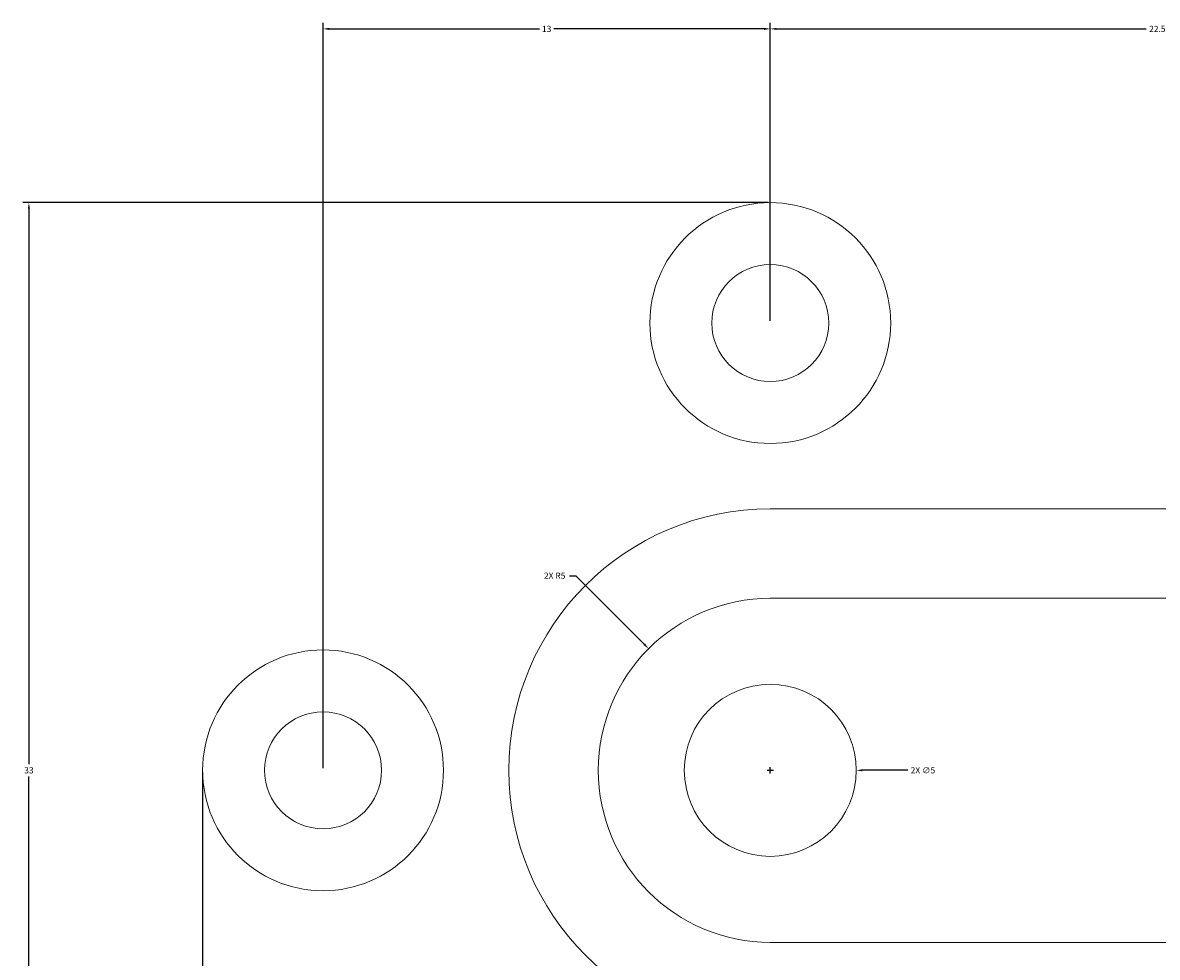
# Model space of a CAD drawing. Units: millimetres. Extents: x 3243.8 to 3309.8, y 1625.7 to 1669.2.
# Tile 2 of 3: x 3243.8 to 3276.8, y 1642 to 1669.2. Entities that reach past the tile are written whole.
import ezdxf

# ---------------------------------------------------------------- set-up
doc = ezdxf.new("R2010")
doc.units = ezdxf.units.MM
doc.layers.add('M-CONS', color=8, linetype='Continuous', lineweight=18)
doc.layers.add('M-DIMS', color=2, linetype='Continuous', lineweight=18)
doc.styles.get("Standard").update_dxf_attribs({"font": 'arial.ttf'})
doc.dimstyles.get("Standard").update_dxf_attribs({"dimtxt": 0.18, "dimasz": 0.18, "dimexe": 0.18, "dimexo": 0.0625, "dimgap": 0.09, "dimtad": 0, "dimtih": 1, "dimtoh": 1, "dimdec": 4, "dimzin": 0, "dimdsep": 46, "dimtxsty": 'Standard', "dimcen": 0.09, "dimadec": 0, "dimazin": 0, "dimtfac": 1, "dimtdec": 4, "dimtofl": 0, "dimtmove": 0, "dimatfit": 3, "dimfxl": 1, "dimtolj": 1, "dimtzin": 0, "dimarcsym": 0})

# ---------------------------------------------------------------- blocks, each defined once
blk = doc.blocks.new('CBORE-7-BORE-3.4')
for centre, radius in [((3.5, 3.5), 3.5), ((3.5, 3.5, -1), 1.7)]:
    blk.add_circle(centre, radius)
blk = doc.blocks.new('*D2')
at = {"layer": 'Defpoints', "color": 0, "transparency": 16777216}
for p in [(3249.045, 1647.47), (3304.545, 1647.47), (3304.545, 1625.92)]:
    blk.add_point(p, dxfattribs=at)
at = {"layer": 'M-DIMS', "color": 0, "lineweight": -2, "transparency": 16777216}
for p, q in [((3249.045, 1647.407), (3249.045, 1625.74)), ((3304.545, 1647.407), (3304.545, 1625.74)), ((3249.225, 1625.92), (3276.47, 1625.92)), ((3304.365, 1625.92), (3277.119, 1625.92))]:
    blk.add_line(p, q, dxfattribs=at)
at = {"layer": 'M-DIMS', "color": 0, "transparency": 16777216}
for points in [[(3249.225, 1625.95), (3249.225, 1625.89), (3249.045, 1625.92)], [(3304.365, 1625.95), (3304.365, 1625.89), (3304.545, 1625.92)]]:
    blk.add_solid(points, dxfattribs=at)
at = {"layer": 'M-DIMS', "color": 0, "transparency": 16777216, "insert": (3276.795, 1625.92), "char_height": 0.18, "attachment_point": 5}
blk.add_mtext('\\A1;55.5', dxfattribs=at)
blk = doc.blocks.new('*D3')
at = {"layer": 'Defpoints', "color": 0, "transparency": 16777216}
for p in [(3243.995, 1663.97), (3265.545, 1663.97), (3265.545, 1630.97)]:
    blk.add_point(p, dxfattribs=at)
at = {"layer": 'M-DIMS', "color": 0, "lineweight": -2, "transparency": 16777216}
for p, q in [((3265.482, 1663.97), (3243.815, 1663.97)), ((3243.995, 1663.79), (3243.995, 1647.652)), ((3243.995, 1631.15), (3243.995, 1647.288)), ((3265.482, 1630.97), (3243.815, 1630.97))]:
    blk.add_line(p, q, dxfattribs=at)
at = {"layer": 'M-DIMS', "color": 0, "transparency": 16777216}
for points in [[(3243.965, 1663.79), (3244.025, 1663.79), (3243.995, 1663.97)], [(3243.965, 1631.15), (3244.025, 1631.15), (3243.995, 1630.97)]]:
    blk.add_solid(points, dxfattribs=at)
at = {"layer": 'M-DIMS', "color": 0, "transparency": 16777216, "insert": (3243.995, 1647.47), "char_height": 0.18, "attachment_point": 5}
blk.add_mtext('\\A1;33', dxfattribs=at)
blk = doc.blocks.new('*D4')
at = {"layer": 'Defpoints', "color": 0, "transparency": 16777216}
for p in [(3265.545, 1669.02), (3265.545, 1660.47), (3252.545, 1647.47)]:
    blk.add_point(p, dxfattribs=at)
at = {"layer": 'M-DIMS', "color": 0, "lineweight": -2, "transparency": 16777216}
for p, q in [((3252.545, 1647.532), (3252.545, 1669.2)), ((3265.545, 1660.532), (3265.545, 1669.2)), ((3252.725, 1669.02), (3258.834, 1669.02)), ((3265.365, 1669.02), (3259.255, 1669.02))]:
    blk.add_line(p, q, dxfattribs=at)
at = {"layer": 'M-DIMS', "color": 0, "transparency": 16777216}
for points in [[(3252.725, 1669.05), (3252.725, 1668.99), (3252.545, 1669.02)], [(3265.365, 1669.05), (3265.365, 1668.99), (3265.545, 1669.02)]]:
    blk.add_solid(points, dxfattribs=at)
at = {"layer": 'M-DIMS', "color": 0, "transparency": 16777216, "insert": (3259.045, 1669.02), "char_height": 0.18, "attachment_point": 5}
blk.add_mtext('\\A1;13', dxfattribs=at)
blk = doc.blocks.new('*D5')
at = {"layer": 'Defpoints', "color": 0, "transparency": 16777216}
for p in [(3288.045, 1669.02), (3265.545, 1660.47), (3288.045, 1660.47)]:
    blk.add_point(p, dxfattribs=at)
at = {"layer": 'M-DIMS', "color": 0, "lineweight": -2, "transparency": 16777216}
for p, q in [((3265.545, 1660.532), (3265.545, 1669.2)), ((3288.045, 1660.532), (3288.045, 1669.2)), ((3265.725, 1669.02), (3276.469, 1669.02)), ((3287.865, 1669.02), (3277.121, 1669.02))]:
    blk.add_line(p, q, dxfattribs=at)
at = {"layer": 'M-DIMS', "color": 0, "transparency": 16777216}
for points in [[(3265.725, 1669.05), (3265.725, 1668.99), (3265.545, 1669.02)], [(3287.865, 1669.05), (3287.865, 1668.99), (3288.045, 1669.02)]]:
    blk.add_solid(points, dxfattribs=at)
at = {"layer": 'M-DIMS', "color": 0, "transparency": 16777216, "insert": (3276.795, 1669.02), "char_height": 0.18, "attachment_point": 5}
blk.add_mtext('\\A1;22.5', dxfattribs=at)
blk = doc.blocks.new('*D8')
at = {"layer": 'Defpoints', "color": 0, "transparency": 16777216}
for p in [(3262.009, 1651.006), (3265.545, 1647.47)]:
    blk.add_point(p, dxfattribs=at)
at = {"layer": 'M-DIMS', "color": 0, "lineweight": -2, "transparency": 16777216}
for p, q in [((3259.708, 1653.127), (3259.888, 1653.127)), ((3259.888, 1653.127), (3261.882, 1651.133)), ((3265.455, 1647.47), (3265.635, 1647.47)), ((3265.545, 1647.38), (3265.545, 1647.56))]:
    blk.add_line(p, q, dxfattribs=at)
at = {"layer": 'M-DIMS', "color": 0, "transparency": 16777216}
blk.add_solid([(3261.903, 1651.154), (3261.861, 1651.112), (3262.009, 1651.006)], dxfattribs=at)
at = {"layer": 'M-DIMS', "color": 0, "transparency": 16777216, "insert": (3259.277, 1653.127), "char_height": 0.18, "attachment_point": 5}
blk.add_mtext('\\A1;2X R5', dxfattribs=at)
blk = doc.blocks.new('*D11')
at = {"layer": 'Defpoints', "color": 0, "transparency": 16777216}
for p in [(3263.045, 1647.47), (3268.045, 1647.47)]:
    blk.add_point(p, dxfattribs=at)
at = {"layer": 'M-DIMS', "color": 0, "lineweight": -2, "transparency": 16777216}
for p, q in [((3265.455, 1647.47), (3265.635, 1647.47)), ((3265.545, 1647.38), (3265.545, 1647.56)), ((3269.545, 1647.47), (3268.225, 1647.47))]:
    blk.add_line(p, q, dxfattribs=at)
at = {"layer": 'M-DIMS', "color": 0, "transparency": 16777216}
blk.add_solid([(3268.225, 1647.5), (3268.225, 1647.44), (3268.045, 1647.47)], dxfattribs=at)
at = {"layer": 'M-DIMS', "color": 0, "transparency": 16777216, "insert": (3269.982, 1647.47), "char_height": 0.18, "attachment_point": 5}
blk.add_mtext('\\A1;2X ∅5', dxfattribs=at)

msp = doc.modelspace()

# ---------------------------------------------------------------- linework, layer by layer
at = {"layer": 'M-CONS'}
for points in [[(3265.545, 1655.07), (3288.045, 1655.07, -1), (3288.045, 1639.87), (3265.545, 1639.87, -1)], [(3288.045, 1652.47), (3265.545, 1652.47, 1), (3265.545, 1642.47), (3288.045, 1642.47, 1)]]:
    msp.add_lwpolyline(points, format="xyb", close=True, dxfattribs=at)
for centre, radius in [((3265.545, 1660.47), 3.5), ((3265.545, 1660.47, -1), 1.7), ((3252.545, 1647.47), 3.5), ((3265.545, 1647.47), 2.5), ((3252.545, 1647.47, -1), 1.7)]:
    msp.add_circle(centre, radius, dxfattribs=at)

# ---------------------------------------------------------------- block references
for p in [(3262.045, 1656.97), (3249.045, 1643.97)]:
    msp.add_blockref('CBORE-7-BORE-3.4', p, dxfattribs=at)

# ---------------------------------------------------------------- dimensions: what is measured, and where the dimension line sits
at = {"layer": 'M-DIMS'}
for base, p1, p2, override, picture, middle in [((3265.545, 1669.02), (3252.545, 1647.47), (3265.545, 1660.47), {"dimdec": 0, "dimlfac": 1, "dimrnd": 0, "dimzin": 0, "dimdsep": 46, "dimlunit": 2}, '*D4', (3259.045, 1669.02)), ((3288.045, 1669.02), (3265.545, 1660.47), (3288.045, 1660.47), {"dimdec": 1, "dimlfac": 1, "dimrnd": 0, "dimzin": 0, "dimdsep": 46, "dimlunit": 2}, '*D5', (3276.795, 1669.02)), ((3304.545, 1625.92), (3249.045, 1647.47), (3304.545, 1647.47), {"dimdec": 1, "dimlfac": 1, "dimrnd": 0, "dimzin": 0, "dimdsep": 46, "dimlunit": 2}, '*D2', (3276.795, 1625.92))]:
    dim = msp.add_linear_dim(base=base, p1=p1, p2=p2, dimstyle='Standard', override=override, dxfattribs=at)
    dim.commit()
    dim.dimension.update_dxf_attribs({"geometry": picture, "text_midpoint": middle})
dim = msp.add_linear_dim(base=(3243.995, 1663.97), p1=(3265.545, 1630.97), p2=(3265.545, 1663.97), angle=90, dimstyle='Standard', override={"dimdec": 0, "dimlfac": 1, "dimrnd": 0, "dimzin": 0, "dimdsep": 46, "dimlunit": 2}, dxfattribs=at)
dim.commit()
dim.dimension.update_dxf_attribs({"geometry": '*D3', "text_midpoint": (3243.995, 1647.47)})
dim = msp.add_radius_dim(center=(3265.545, 1647.47), mpoint=(3262.009, 1651.006), text='2X <>', dimstyle='Standard', override={"dimdec": 0, "dimlfac": 1, "dimrnd": 0, "dimzin": 0, "dimdsep": 46, "dimlunit": 2}, dxfattribs=at)
dim.commit()
dim.dimension.update_dxf_attribs({"geometry": '*D8', "text_midpoint": (3259.277, 1653.127), "dimtype": 164})
dim = msp.add_diameter_dim_2p(p1=(3263.045, 1647.47), p2=(3268.045, 1647.47), text='2X <>', dimstyle='Standard', override={"dimdec": 0, "dimlfac": 1, "dimrnd": 0, "dimzin": 0, "dimdsep": 46, "dimlunit": 2}, dxfattribs=at)
dim.commit()
dim.dimension.update_dxf_attribs({"geometry": '*D11', "text_midpoint": (3269.545, 1647.47), "dimtype": 163})

doc.saveas('drawing.dxf')
